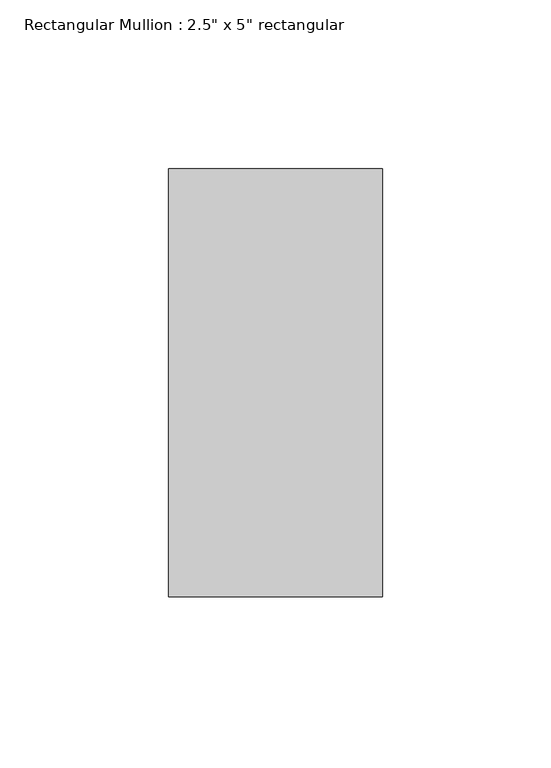
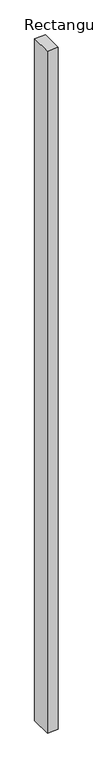
"""IFC4 building model written with IfcOpenShell, lengths in millimetres: member geometry."""

from ifc_helpers import new_model, si_unit, frame, origin, place, context, project, spatial, polyline, outline, extrude, source, transform, mapped, element, save


def member_147bebee(model_context):
    return source(origin(), model_context, "Body", "SweptSolid", [
        extrude(outline(polyline([(0.0, 63.5), (0.0, -63.5), (-63.5, -63.5), (-63.5, 63.5), (0.0, 63.5)])), frame((0.0, 0.0, -4191.0), z_axis=(0.0, 0.0, 1.0), x_axis=(1.0, 0.0, 0.0)), (0.0, 0.0, 1.0), 4191.0),
    ])


if __name__ == "__main__":
    model = new_model("IFC4")
    model_context = context("Model", 3, world=origin())
    ifc_project = project(units=[si_unit("LENGTHUNIT", "METRE", prefix="MILLI")], contexts=[model_context])
    site = spatial("IfcSite", under=ifc_project)
    building = spatial("IfcBuilding", under=site)
    placement = place(None, origin())
    member_shape = member_147bebee(model_context)
    element("IfcMember", 1, ObjectType="Rectangular Mullion : 2.5\" x 5\" rectangular", at=placement, inside=building, context=model_context, shape_type="MappedRepresentation", body=[
        mapped(member_shape, transform((0.0, 0.0, 0.0), x_axis=(1.0, 0.0, 0.0), y_axis=(0.0, 1.0, 0.0), z_axis=(0.0, 0.0, 1.0))),
    ])
    save(model, "model.ifc")

# Revit data of these elements
# Type "Rectangular Mullion : 2.5\" x 5\" rectangular"
#   built-in parameter 1007304 = 0.416667 (stored number, unit not read)
#   built-in parameter 1007301 = 0.104167 (stored number, unit not read)
#   built-in parameter 1007300 = 0.104167 (stored number, unit not read)
# Element 1 (IfcMember, "Rectangular Mullion : 2.5\" x 5\" rectangular")
#   Materials on its faces: "Aluminum"
# Materials
#   "Aluminum": class "Metal", colour RGB 247 247 247, transparency 0, Description = "Aluminum 6061", Cost = 0
